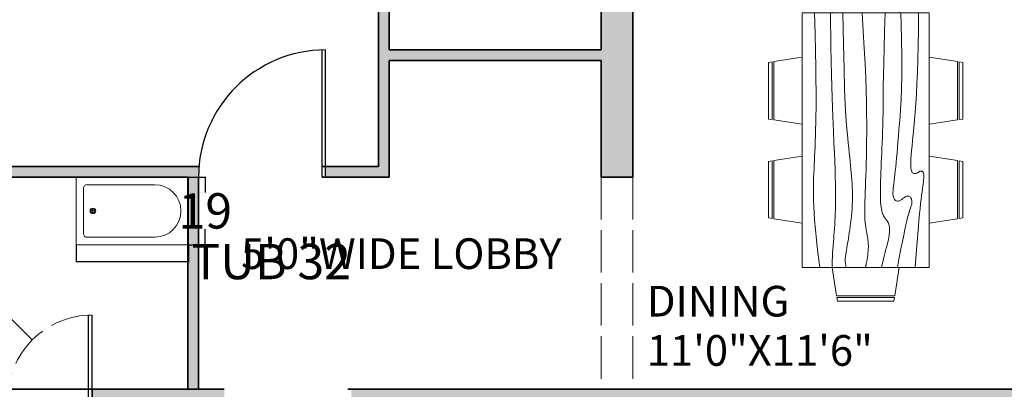
# Model space of a CAD drawing. Units: inches. Extents: x 215 to 969, y -612 to 418.
# Tile 6 of 8: x 405 to 684, y 109 to 214. Entities that reach past the tile are written whole.
import ezdxf

# ---------------------------------------------------------------- set-up
doc = ezdxf.new("R2010")
doc.units = ezdxf.units.IN
doc.header["$MEASUREMENT"] = 0
doc.linetypes.add('ACAD_ISO02W100', pattern=[15, 12, -3])
for name, color, linetype, lineweight in [('A-ANNO-DIMS', 2, 'Continuous', 18), ('A-AREA-IDEN', 7, 'Continuous', 18), ('A-DOOR', 3, 'Continuous', 25), ('A-DOOR-SWNG', 3, 'ACAD_ISO02W100', 13), ('A-FLOR-FIXT', 9, 'Continuous', 18), ('A-FURN', 8, 'Continuous', 18), ('A-WALL', 7, 'Continuous', 35), ('A-WALL-OVHD', 7, 'ACAD_ISO02W100', 18)]:
    doc.layers.add(name, color=color, linetype=linetype, lineweight=lineweight)
doc.layers.add('A-WALL-PATT', color=252, linetype='Continuous', lineweight=13, true_color=0x939598)
doc.styles.get("Standard").update_dxf_attribs({"font": 'arial.ttf'})
doc.dimstyles.get("Standard").update_dxf_attribs({"dimtxt": 10, "dimasz": 0.18, "dimexe": 0.18, "dimexo": 0.0625, "dimgap": 0.09, "dimtad": 0, "dimtih": 1, "dimtoh": 1, "dimdec": 0, "dimzin": 0, "dimdsep": 46, "dimlunit": 3, "dimtxsty": 'Standard', "dimcen": 0.09, "dimadec": 0, "dimazin": 0, "dimtfac": 1, "dimtdec": 0, "dimtofl": 0, "dimtmove": 0, "dimatfit": 3, "dimfxl": 1, "dimtolj": 1, "dimtzin": 0, "dimarcsym": 0})

# ---------------------------------------------------------------- blocks, each defined once
blk = doc.blocks.new('Dining Set - 36 x 72 in.')
for p, q in [((-22.2343, 26.00059), (-23.4847, 17.99762)), ((-22.2304, 26), (-5.7608, 26)), ((-22, 27.5), (-22.1562, 26.50042)), ((-5.8416, 26.5), (-22.1534, 26.5)), ((-22, 27.5), (-6, 27.5)), ((-5.8437, 26.49966), (-6, 27.5)), ((-4.5152, 17.99762), (-5.7655, 25.99926)), ((5.7657, 26.00059), (4.5153, 17.99762)), ((5.7696, 26), (22.2392, 26)), ((6, 27.5), (5.8438, 26.50042)), ((22.1584, 26.5), (5.8466, 26.5)), ((6, 27.5), (22, 27.5)), ((22.1563, 26.49966), (22, 27.5)), ((23.4848, 17.99762), (22.2345, 25.99926)), ((36, 18), (-36, 18)), ((-36, 18), (-36, -18)), ((36, -18), (36, 18)), ((-44.0006, 8.23428), (-35.9976, 9.48474)), ((44.0006, 8.23428), (35.9976, 9.48474)), ((-45.5, 8), (-44.5004, 8.15617)), ((-45.5, 8), (-45.5, -8)), ((-44.5, -8.15843), (-44.5, 8.15338)), ((-44, 8.23041), (-44, -8.23915)), ((44, 8.23041), (44, -8.23915)), ((44.5, -8.15843), (44.5, 8.15338)), ((45.5, 8), (44.5005, 8.15617)), ((45.5, 8), (45.5, -8)), ((-44.4997, -8.15631), (-45.5, -8)), ((-35.9976, -9.48476), (-43.9993, -8.2345)), ((35.9976, -9.48476), (43.9993, -8.2345)), ((44.4997, -8.15631), (45.5, -8)), ((-36, -18), (36, -18)), ((-22.2343, -26.0006), (-23.4847, -17.99762)), ((-4.5152, -17.99762), (-5.7655, -25.99928)), ((5.7657, -26.0006), (4.5153, -17.99762)), ((23.4848, -17.99762), (22.2345, -25.99928)), ((-22.2304, -26), (-5.7608, -26)), ((-22, -27.5), (-22.1562, -26.50044)), ((-5.8416, -26.5), (-22.1534, -26.5)), ((-22, -27.5), (-6, -27.5)), ((-5.8437, -26.49967), (-6, -27.5)), ((5.7696, -26), (22.2392, -26)), ((6, -27.5), (5.8438, -26.50044)), ((22.1584, -26.5), (5.8466, -26.5)), ((6, -27.5), (22, -27.5)), ((22.1563, -26.49967), (22, -27.5))]:
    blk.add_line(p, q)
for points in [[(-36, 15), (-31.1772, 14.97754), (-26.8079, 14.91406), (-22.8538, 14.81543), (-19.276, 14.6875), (-16.0362, 14.53613), (-13.0957, 14.36718), (-10.4159, 14.18652), (-7.9583, 14), (-5.6904, 13.81315), (-3.6035, 13.63021), (-1.6954, 13.45508), (0.0365, 13.29166), (1.5945, 13.14388), (2.9811, 13.01562), (4.1988, 12.9108), (5.25, 12.83333), (6.1393, 12.78613), (6.8802, 12.76823), (7.4883, 12.77767), (7.9792, 12.8125), (8.3685, 12.87077), (8.6719, 12.95052), (8.9049, 13.0498), (9.0833, 13.16666), (9.2205, 13.29899), (9.3216, 13.44401), (9.3895, 13.59879), (9.4271, 13.76041), (9.4373, 13.92594), (9.4232, 14.09245), (9.3875, 14.257), (9.3333, 14.41666), (9.2638, 14.56917), (9.1836, 14.71484), (9.0975, 14.85465), (9.0104, 14.98958), (8.9272, 15.1206), (8.8529, 15.2487), (8.7922, 15.37483), (8.75, 15.5), (8.7305, 15.62467), (8.7344, 15.74739), (8.7617, 15.86621), (8.8125, 15.97916), (8.8867, 16.08431), (8.9844, 16.17968), (9.1055, 16.26334), (9.25, 16.33333), (9.4189, 16.38802), (9.6172, 16.42708), (9.8506, 16.45052), (10.125, 16.45833), (10.4463, 16.45052), (10.8203, 16.42708), (11.2529, 16.38802), (11.75, 16.33333), (12.3184, 16.26318), (12.9694, 16.17838), (13.7151, 16.07991), (14.5677, 15.96875), (15.5395, 15.84586), (16.6426, 15.71224), (17.8893, 15.56884), (19.2917, 15.41666), (20.859, 15.25667), (22.5879, 15.08984), (24.4721, 14.91715), (26.5052, 14.73958), (28.6809, 14.5581), (30.9929, 14.3737), (33.4347, 14.18733), (36, 14)], [(-36, 10), (-28.9766, 10.14274), (-23.1725, 10.20442), (-18.4241, 10.19775), (-14.5677, 10.13541), (-11.4399, 10.03011), (-8.877, 9.89453), (-6.7154, 9.74137), (-4.7917, 9.58333), (-2.9698, 9.43082), (-1.2246, 9.28515), (0.4415, 9.14534), (2.026, 9.01041), (3.5266, 8.87939), (4.9408, 8.7513), (6.266, 8.62516), (7.5, 8.5), (8.6411, 8.37549), (9.6914, 8.2539), (10.6538, 8.13818), (11.5312, 8.03125), (12.3267, 7.93603), (13.043, 7.85547), (13.6831, 7.79248), (14.25, 7.75), (14.7471, 7.7303), (15.1797, 7.73307), (15.5537, 7.75732), (15.875, 7.80208), (16.1494, 7.86637), (16.3828, 7.94922), (16.5811, 8.04964), (16.75, 8.16666), (16.8944, 8.29915), (17.0143, 8.44531), (17.1089, 8.60319), (17.1771, 8.77083), (17.218, 8.94629), (17.2305, 9.1276), (17.2137, 9.31282), (17.1667, 9.5), (17.0895, 9.6875), (16.987, 9.875), (16.8649, 10.0625), (16.7292, 10.25), (16.5856, 10.4375), (16.4401, 10.625), (16.2985, 10.8125), (16.1667, 11), (16.05, 11.18733), (15.9518, 11.3737), (15.8752, 11.5581), (15.8229, 11.73958), (15.798, 11.91715), (15.8034, 12.08984), (15.842, 12.25667), (15.9167, 12.41666), (16.0295, 12.56836), (16.1784, 12.70833), (16.3605, 12.83268), (16.5729, 12.9375), (16.8127, 13.01888), (17.0768, 13.07291), (17.3625, 13.0957), (17.6667, 13.08333), (17.9894, 13.03312), (18.3418, 12.94726), (18.7382, 12.82918), (19.1927, 12.68229), (19.7195, 12.51001), (20.3327, 12.31575), (21.0465, 12.10294), (21.875, 11.875), (22.8357, 11.63354), (23.959, 11.37304), (25.2786, 11.08618), (26.8282, 10.76562), (28.6414, 10.40405), (30.752, 9.99414), (33.1936, 9.52856), (36, 9)], [(-36, 5.5), (-30.7157, 5.3348), (-26.069, 5.20963), (-21.9946, 5.11767), (-18.4271, 5.05208), (-15.3009, 5.00602), (-12.5508, 4.97265), (-10.1112, 4.94515), (-7.9167, 4.91666), (-5.909, 4.88167), (-4.0586, 4.83984), (-2.3429, 4.79215), (-0.7396, 4.73958), (0.7739, 4.6831), (2.22, 4.6237), (3.6213, 4.56233), (5, 4.5), (6.373, 4.43782), (7.7344, 4.3776), (9.0723, 4.32129), (10.375, 4.27083), (11.6309, 4.22819), (12.8281, 4.19531), (13.9551, 4.17415), (15, 4.16666), (15.954, 4.17448), (16.819, 4.19791), (17.6001, 4.23698), (18.3021, 4.29166), (18.9299, 4.36198), (19.4883, 4.44791), (19.9823, 4.54948), (20.4167, 4.66666), (20.7969, 4.79899), (21.1302, 4.94401), (21.4245, 5.09879), (21.6875, 5.26041), (21.9271, 5.42594), (22.1511, 5.59245), (22.3672, 5.757), (22.5834, 5.91666), (22.8065, 6.06868), (23.0404, 6.21093), (23.2879, 6.34147), (23.5521, 6.45833), (23.8358, 6.55957), (24.142, 6.64323), (24.4735, 6.70735), (24.8334, 6.75), (25.2235, 6.76969), (25.642, 6.76692), (26.0858, 6.74267), (26.5521, 6.69791), (27.0379, 6.63362), (27.5404, 6.55078), (28.0565, 6.45036), (28.5834, 6.33333), (29.1242, 6.19987), (29.7071, 6.04687), (30.3661, 5.87044), (31.1354, 5.66666), (32.0493, 5.43164), (33.142, 5.16146), (34.4475, 4.85221), (36, 4.5)], [(-36, -1), (-30.7915, -0.6591), (-26.0195, -0.38216), (-21.6519, -0.16284), (-17.6563, 0.00521), (-14.0005, 0.12833), (-10.6523, 0.21289), (-7.5796, 0.26522), (-4.75, 0.29166), (-2.134, 0.29793), (0.2878, 0.28711), (2.5317, 0.26163), (4.6146, 0.22396), (6.5529, 0.17651), (8.3633, 0.12174), (10.0623, 0.06209), (11.6667, 0), (13.1899, -0.06201), (14.6341, -0.1211), (15.9982, -0.17432), (17.2813, -0.21875), (18.4823, -0.25147), (19.6003, -0.26953), (20.6343, -0.27002), (21.5834, -0.25), (22.4481, -0.20768), (23.2357, -0.14584), (23.9549, -0.06836), (24.6146, 0.02083), (25.2235, 0.11784), (25.7904, 0.21875), (26.3241, 0.31966), (26.8334, 0.41666), (27.3265, 0.50618), (27.8099, 0.58593), (28.2894, 0.65397), (28.7709, 0.70833), (29.2601, 0.74707), (29.763, 0.76823), (30.2855, 0.76985), (30.8334, 0.75), (31.4088, 0.70784), (31.9994, 0.64713), (32.589, 0.57275), (33.1615, 0.48958), (33.7008, 0.4025), (34.1908, 0.3164), (34.6153, 0.23616), (34.9584, 0.16666), (35.2099, 0.11165), (35.3848, 0.07031), (35.504, 0.04069), (35.5886, 0.02083), (35.6594, 0.00879), (35.7377, 0.0026), (35.8442, 0.00032), (36, 0)], [(-36, -6.5), (-27.1843, -6.31267), (-20.084, -6.1263), (-14.469, -5.9419), (-10.1094, -5.76042), (-6.7752, -5.58285), (-4.2363, -5.41016), (-2.2629, -5.24333), (-0.625, -5.08334), (0.8708, -4.93099), (2.2715, -4.78646), (3.5872, -4.64974), (4.8281, -4.52084), (6.0046, -4.39974), (7.127, -4.28646), (8.2053, -4.18099), (9.25, -4.08334), (10.2705, -3.99382), (11.2734, -3.91407), (12.2647, -3.84603), (13.25, -3.79167), (14.2354, -3.75293), (15.2266, -3.73177), (16.2295, -3.73015), (17.25, -3.75), (18.2912, -3.79248), (19.3451, -3.85547), (20.4009, -3.93604), (21.4479, -4.03125), (22.4754, -4.13819), (23.4727, -4.25391), (24.4289, -4.37549), (25.3334, -4.5), (26.1785, -4.62492), (26.9694, -4.74935), (27.7145, -4.87281), (28.4219, -4.99479), (29.1, -5.11483), (29.7572, -5.23242), (30.4016, -5.34709), (31.0417, -5.45834), (31.6837, -5.56437), (32.3262, -5.65821), (32.9658, -5.73153), (33.599, -5.77604), (34.2224, -5.78345), (34.8327, -5.74545), (35.4264, -5.65373), (36, -5.5)], [(-36, -10), (-26.4022, -9.81299), (-18.4675, -9.62891), (-11.9839, -9.45069), (-6.7396, -9.28125), (-2.5226, -9.12354), (0.8789, -8.98047), (3.6769, -8.85498), (6.0833, -8.75), (8.2767, -8.66765), (10.3021, -8.60677), (12.1712, -8.56543), (13.8958, -8.54167), (15.4876, -8.53353), (16.9583, -8.53907), (18.3197, -8.55632), (19.5834, -8.58334), (20.7616, -8.61841), (21.8685, -8.66081), (22.9188, -8.71004), (23.9271, -8.76563), (24.9081, -8.82707), (25.8763, -8.89388), (26.8465, -8.96558), (27.8334, -9.04167), (28.8474, -9.12118), (29.8828, -9.20117), (30.93, -9.27824), (31.9792, -9.34896), (33.0205, -9.40991), (34.0443, -9.45768), (35.0407, -9.48885), (36, -9.5)], [(-36, -14.5), (-30.0881, -14.33513), (-25.0332, -14.21224), (-20.7312, -14.12647), (-17.0781, -14.07292), (-13.97, -14.04671), (-11.3027, -14.04297), (-8.9724, -14.05681), (-6.875, -14.08334), (-4.9224, -14.11833), (-3.0905, -14.16016), (-1.3709, -14.20785), (0.2448, -14.26042), (1.7647, -14.3169), (3.1973, -14.3763), (4.5507, -14.43767), (5.8333, -14.5), (7.0554, -14.5621), (8.235, -14.62175), (9.3922, -14.67652), (10.5469, -14.72396), (11.7192, -14.76164), (12.929, -14.78711), (14.1965, -14.79794), (15.5417, -14.79167), (16.9933, -14.76424), (18.6152, -14.70508), (20.4804, -14.60197), (22.6615, -14.44271), (25.2312, -14.21509), (28.2624, -13.9069), (31.8277, -13.50594), (36, -13)]]:
    blk.add_lwpolyline(points)
blk = doc.blocks.new('Bath Tub - 26 x 60 in.')
for p, q in [((8, -18), (10, -18)), ((9, -17), (9, -19))]:
    blk.add_line(p, q)
blk.add_lwpolyline([(0, -36), (0, 0), (60, 0), (60, -36)], close=True)
for points in [[(6, -4), (42, -4)], [(4, -30), (4, -6)], [(42, -32), (6, -32)]]:
    blk.add_lwpolyline(points)
for radius in [1.5, 1]:
    blk.add_circle((9, -18), radius)
for centre, radius, start, end in [((5.75, -5.75), 1.77, 81.8699, 188.1301), ((42, -18), 14, 270, 90), ((5.75, -30.25), 1.77, 171.8699, 278.1301)]:
    blk.add_arc(centre, radius, start, end)
blk = doc.blocks.new('DOOR-SINGLE-36')
for p, q in [((35, 0), (35, 36)), ((36, 0), (36, 36)), ((35, 0), (36, 0))]:
    blk.add_line(p, q)
blk.add_arc((36, 0), 36, 90, 180)
blk = doc.blocks.new('*D31')
at = {"layer": 'A-ANNO-DIMS', "color": 0, "lineweight": -2, "transparency": 16777216}
for p, q in [((420.68, 150.06), (420.68, 145.17)), ((452.5, 150.06), (452.5, 145.17)), ((420.86, 145.35), (452.32, 145.35)), ((452.5, 145.35), (452.68, 145.35))]:
    blk.add_line(p, q, dxfattribs=at)
at = {"layer": 'A-ANNO-DIMS', "color": 0, "transparency": 16777216}
for points in [[(420.86, 145.38), (420.86, 145.32), (420.68, 145.35)], [(452.32, 145.38), (452.32, 145.32), (452.5, 145.35)]]:
    blk.add_solid(points, dxfattribs=at)
at = {"layer": 'Defpoints', "color": 0, "transparency": 16777216}
for p in [(420.68, 150.12), (452.5, 150.12), (452.5, 145.35)]:
    blk.add_point(p, dxfattribs=at)
at = {"layer": 'A-ANNO-DIMS', "color": 0, "transparency": 16777216, "insert": (475.92, 145.35), "char_height": 10, "attachment_point": 5}
blk.add_mtext('\\A1;TUB 32', dxfattribs=at)
blk = doc.blocks.new('*D32')
at = {"layer": 'A-ANNO-DIMS', "color": 0, "lineweight": -2, "transparency": 16777216}
for p, q in [((452.57, 169.21), (457.46, 169.21)), ((457.28, 169.03), (457.28, 164.86)), ((457.28, 150.3), (457.28, 154.47)), ((452.57, 150.12), (457.46, 150.12))]:
    blk.add_line(p, q, dxfattribs=at)
at = {"layer": 'A-ANNO-DIMS', "color": 0, "transparency": 16777216}
for points in [[(457.25, 169.03), (457.31, 169.03), (457.28, 169.21)], [(457.25, 150.3), (457.31, 150.3), (457.28, 150.12)]]:
    blk.add_solid(points, dxfattribs=at)
at = {"layer": 'Defpoints', "color": 0, "transparency": 16777216}
for p in [(452.5, 169.21), (457.28, 169.21), (452.5, 150.12)]:
    blk.add_point(p, dxfattribs=at)
at = {"layer": 'A-ANNO-DIMS', "color": 0, "transparency": 16777216, "insert": (457.28, 159.67), "char_height": 10, "attachment_point": 5}
blk.add_mtext('\\A1;19', dxfattribs=at)
blk = doc.blocks.new('*D76')
at = {"layer": 'A-ANNO-DIMS', "color": 0, "lineweight": -2, "transparency": 16777216}
for p, q in [((569.29, 365.5), (243.77, 365.5)), ((243.95, 365.32), (243.95, -91.71)), ((243.95, -559.13), (243.95, -102.1)), ((454.66, -559.31), (243.77, -559.31))]:
    blk.add_line(p, q, dxfattribs=at)
at = {"layer": 'A-ANNO-DIMS', "color": 0, "transparency": 16777216}
for points in [[(243.92, 365.32), (243.98, 365.32), (243.95, 365.5)], [(243.92, -559.13), (243.98, -559.13), (243.95, -559.31)]]:
    blk.add_solid(points, dxfattribs=at)
at = {"layer": 'Defpoints', "color": 0, "transparency": 16777216}
for p in [(569.35, 365.5), (243.95, -559.31), (454.72, -559.31)]:
    blk.add_point(p, dxfattribs=at)
at = {"layer": 'A-ANNO-DIMS', "color": 0, "transparency": 16777216, "insert": (243.95, -96.91), "char_height": 10, "attachment_point": 5}
blk.add_mtext('\\A1;924.8', dxfattribs=at)
blk = doc.blocks.new('*D85')
at = {"layer": 'A-ANNO-DIMS', "color": 0, "lineweight": -2, "transparency": 16777216}
for p, q in [((397.96, 133.26), (398.14, 133.26)), ((398.14, 133.26), (408.16, 123.3)), ((425.11, 106.37), (425.29, 106.37)), ((425.2, 106.28), (425.2, 106.46))]:
    blk.add_line(p, q, dxfattribs=at)
at = {"layer": 'A-ANNO-DIMS', "color": 0, "transparency": 16777216}
blk.add_solid([(408.18, 123.32), (408.14, 123.28), (408.29, 123.18)], dxfattribs=at)
at = {"layer": 'Defpoints', "color": 0, "transparency": 16777216}
for p in [(408.29, 123.18), (425.2, 106.37)]:
    blk.add_point(p, dxfattribs=at)
at = {"layer": 'A-ANNO-DIMS', "color": 0, "transparency": 16777216, "insert": (372.32, 133.26), "char_height": 10, "attachment_point": 5}
blk.add_mtext('\\A1;R23.847', dxfattribs=at)

msp = doc.modelspace()

# ---------------------------------------------------------------- hatches: boundary and pattern name
at = {"layer": 'A-WALL-PATT'}
h = msp.add_hatch(color=256, dxfattribs=at)
h.dxf.hatch_style = 1
h.paths.add_polyline_path([(764.0736, 322.2135), (569.3535, 322.2135), (565.0643, 322.2135), (565.0643, 313.2135), (569.3535, 313.2135), (569.3535, 205.2135), (509.3535, 205.2135), (509.3535, 247.2592), (506.3535, 247.2592), (506.3535, 172.2135), (491.3535, 172.2135), (491.3535, 169.2135), (509.3535, 169.2135), (509.3535, 202.2135), (569.3535, 202.2135), (569.3535, 169.2135), (578.3535, 169.2135), (578.3535, 205.2135), (578.3535, 237.2135), (615.7789, 237.2135), (615.7789, 246.2135), (578.3535, 246.2135), (578.3535, 313.2135), (710.3535, 313.2135), (710.3535, 246.2135), (710.3535, 211.3874), (719.3535, 211.3874), (719.3535, 295.2135), (719.3535, 313.2135), (764.0736, 313.2135)])
h.paths.add_polyline_path([(879.3535, 322.2135), (811.6486, 322.2135), (811.6486, 313.2135), (870.3535, 313.2135), (870.3535, 215.3905, -0.06325422), (879.3535, 216.5337), (879.3535, 313.2135)])
h.paths.add_polyline_path([(879.3535, 157.2135), (879.3535, 180.5337), (870.3535, 180.5337), (870.3535, 157.2135), (719.3535, 157.2135), (710.3535, 157.2135), (710.3535, 148.2135), (719.3535, 148.2135), (870.3535, 148.2135), (870.3535, 16.2135), (838.4933, 16.2135), (838.4933, 13.2135), (870.3535, 13.2135), (870.3535, -37.7865), (844.0345, -37.7865), (844.0345, -46.7865), (870.3535, -46.7865), (879.3535, -46.7865), (879.3535, -37.7865), (879.3535, 137.613)])
h.paths.add_polyline_path([(710.3535, 246.2135), (663.4146, 246.2135), (663.4146, 237.2135), (710.3535, 237.2135)], flags=17)
h.paths.add_polyline_path([(541.2942, 322.2135), (509.3535, 322.2135), (468.3222, 322.2135), (468.3222, 313.2135), (500.3535, 313.2135), (509.3535, 313.2135), (541.2942, 313.2135)])
h.paths.add_polyline_path([(509.3535, 313.2135), (503.3535, 313.2135), (503.3535, 277.5241, -0.04952579), (509.3535, 277.4203)], flags=17)
h.paths.add_polyline_path([(420.2828, 322.2135), (335.3535, 322.2135), (335.3535, 235.2487), (344.3535, 235.2487), (344.3535, 284.1885), (344.3535, 313.2135), (420.2828, 313.2135)])
h.paths.add_polyline_path([(335.3535, 181.2135), (290.3535, 181.2135), (290.3535, 103.2135), (335.3535, 103.2135), (335.3535, 112.2135), (299.3535, 112.2135), (299.3535, 129.1615), (299.3535, 172.2135), (335.3535, 172.2135)])
h.paths.add_polyline_path([(344.3535, 199.3097), (335.3535, 199.3097), (335.3535, 172.2135), (335.3535, 157.3369), (344.3535, 157.3369), (344.3535, 169.2135), (452.3535, 169.2135), (452.5037, 169.2135), (452.5037, 150.1199), (452.3535, 109.2135), (455.3535, 109.2135), (455.3535, 169.2135, -0.02086055), (455.4787, 172.2135), (344.3535, 172.2135)])
h.paths.add_polyline_path([(344.3535, 133.3441), (335.3535, 133.3441), (335.3535, 77.89), (344.3535, 77.89), (344.3535, 103.2135), (401.3556, 103.2135), (401.3556, 109.2135), (344.3535, 109.2135)])
h.paths.add_polyline_path([(462.6362, 109.2135), (443.0437, 109.2135), (425.2018, 109.2135), (425.2018, 106.2135), (452.3535, 106.2135), (462.7615, 106.2135, -0.02086055)])
h.paths.add_polyline_path([(540.3535, 106.2135), (684.3535, 106.2135), (684.3535, 35.7135), (687.3535, 35.7135), (687.3535, 56.1856), (693.3535, 56.1856), (693.3535, 109.2135), (540.3535, 109.2135), (531.3535, 109.2135), (498.6362, 109.2135), (498.6362, 106.2135), (531.3535, 106.2135), (531.3535, -37.7865), (507.9524, -37.7865), (507.9524, -46.7865), (610.6038, -46.7865), (610.6038, -37.7865), (540.3535, -37.7865)])
h.paths.add_polyline_path([(578.3535, 358.6622), (555.879, 358.6622), (555.879, 349.6622), (569.3535, 349.6622), (569.3535, 322.2135), (578.3535, 322.2135)])
h.paths.add_polyline_path([(525.962, 358.6622), (503.3535, 358.6622), (503.3535, 322.2135), (509.3535, 322.2135), (509.3535, 349.6622), (525.962, 349.6622)])
h.paths.add_polyline_path([(344.3535, 30.022), (335.3535, 30.022), (335.3535, -37.7865), (335.3535, -46.7865), (484.3302, -46.7865), (484.3302, -37.7865), (344.3535, -37.7865)])
h.paths.add_polyline_path([(719.1188, -37.7865), (698.4193, -37.7865), (693.3535, -37.7865), (693.3535, 7.424, -0.07717369), (684.3535, 6.0404), (684.3535, -37.7865), (658.8269, -37.7865), (658.8269, -46.7865), (684.3535, -46.7865), (684.3535, -82.7865), (693.3535, -82.7865), (704.1236, -82.7865), (704.1236, -78.0462), (693.3535, -78.0462), (693.3535, -46.7865), (719.1188, -46.7865)])
h.paths.add_polyline_path([(684.3535, -14.2202), (669.6716, -14.2202), (669.6716, -16.6044, -0.23606798), (667.6716, -17.6044), (667.6716, -18.6044, -0.11764706), (650.6716, -18.6044), (650.6716, -17.6044, -0.23606798), (648.6716, -16.6044), (648.6716, -14.2202), (603.0565, -14.2202), (603.0565, -37.7865), (684.3535, -37.7865)], flags=17)
h.paths.add_polyline_path([(665.6716, -14.2202), (652.6716, -14.2202), (652.6716, -16.6044, -0.23606798), (650.6716, -17.6044), (650.6716, -18.6044, 0.11764706), (667.6716, -18.6044), (667.6716, -17.6044, -0.23606798), (665.6716, -16.6044)], flags=16)
h.paths.add_polyline_path([(786.7385, -37.7865), (755.3535, -37.7865), (755.3535, 13.2135), (769.0808, 13.2135), (769.0808, 16.2135), (755.3535, 16.2135), (755.3535, 73.2135), (753.3535, 73.2135), (693.3535, 73.2135), (693.3535, 70.2135), (753.3535, 70.2135), (753.3535, -37.7865), (743.3062, -37.7865), (743.3062, -46.7865), (781.7385, -46.7865), (781.7385, -82.7865), (786.7385, -82.7865), (786.7385, -82.3744), (786.7385, -46.7865)])
h.paths.add_polyline_path([(844.0345, -37.7865), (786.7385, -37.7865), (786.7385, -46.7865), (844.0345, -46.7865)], flags=17)
h.paths.add_polyline_path([(781.7385, -78.0462), (704.1236, -78.0462), (704.1236, -82.7865), (781.7385, -82.7865)], flags=17)
h.paths.add_polyline_path([(344.3535, -46.7865), (335.3535, -46.7865), (335.3535, -166.4525), (344.3535, -166.4525)])
h.paths.add_polyline_path([(382.6632, 103.2135), (344.3535, 103.2135), (344.3535, 77.89), (344.3535, 32.7135), (363.5083, 32.7135), (382.6632, 32.7135)])
h.paths.add_polyline_path([(879.3535, -46.7865), (870.3535, -46.7865), (870.3535, -166.4525), (879.3535, -166.4525)])
h.paths.add_polyline_path([(879.3535, -166.4525), (799.4745, -166.4525), (799.4745, -175.4525), (855.3535, -175.4525), (870.3535, -175.4525), (870.3535, -192.5449), (879.3535, -192.5449), (879.3535, -175.4525)])
h.paths.add_polyline_path([(763.1775, -166.4525), (655.7214, -166.4525), (655.7214, -175.4525), (763.1775, -175.4525)])
h.paths.add_polyline_path([(619.8538, -166.4525), (550.8369, -166.4525), (550.8369, -175.4525), (619.8538, -175.4525)])
h.paths.add_polyline_path([(527.1282, -166.4525), (427.0819, -166.4525), (427.0819, -175.4525), (527.1282, -175.4525)])
h.paths.add_polyline_path([(391.4021, -166.4525), (335.3535, -166.4525), (335.3535, -175.4525), (335.3535, -236.0109), (344.3535, -236.0109), (344.3535, -187.5037), (344.3535, -175.4525), (391.4021, -175.4525)])
h.paths.add_polyline_path([(344.3535, -271.9249), (335.3535, -271.9249), (335.3535, -331.0209), (344.3535, -331.0209), (344.3535, -314.4525), (412.4218, -314.4525, -0.02503209), (412.3073, -311.4525), (344.3535, -311.4525)])
h.paths.add_polyline_path([(470.1954, -311.4525), (442.3073, -311.4525), (442.3073, -314.4525), (470.0702, -314.4525, -0.02086055)])
h.paths.add_polyline_path([(455.3535, -314.4525), (452.3535, -314.4525), (452.3535, -374.4525), (455.3535, -374.4525)])
h.paths.add_polyline_path([(579.3535, -241.4072), (519.3535, -241.4072), (519.3535, -283.4525), (579.3535, -283.4525)])
h.paths.add_polyline_path([(516.5043, -281.1089), (584.3098, -281.1089), (584.3098, -264.0138), (516.5043, -264.0138)], flags=9)
h.paths.add_polyline_path([(516.4662, -263.2183), (581.1504, -263.2183), (581.1504, -245.8948), (516.4662, -245.8948)], flags=9)

# ---------------------------------------------------------------- linework, layer by layer
at = {"layer": 'A-DOOR'}
for p, q in [((424.2018, 106.2135), (424.2018, 130.2135)), ((425.2018, 106.2135), (425.2018, 130.2135)), ((425.2018, 109.2135), (425.2018, 106.2135))]:
    msp.add_line(p, q, dxfattribs=at)
at = {"layer": 'A-DOOR-SWNG'}
msp.add_arc((425.2018, 106.3669), 23.8466, 90, 180.368506, dxfattribs=at)
at = {"layer": 'A-WALL'}
for p, q in [((509.3535, 205.2135), (509.3535, 313.2135)), ((569.3535, 313.2135), (569.3535, 205.2135)), ((506.3535, 172.2135), (506.3535, 248.2592)), ((578.3535, 237.2135), (578.3535, 205.2135)), ((569.3535, 205.2135), (509.3535, 205.2135)), ((578.3535, 169.2135), (578.3535, 205.2135)), ((509.3535, 169.2135), (509.3535, 202.2135)), ((569.3535, 202.2135), (509.3535, 202.2135)), ((569.3535, 202.2135), (569.3535, 169.2135)), ((344.3535, 172.2135), (455.4787, 172.2135)), ((490.3535, 172.2135), (506.3535, 172.2135)), ((344.3535, 169.2135), (452.3535, 169.2135)), ((452.3535, 109.2135), (452.3535, 169.2135)), ((455.3535, 109.2135), (455.3535, 169.2135)), ((490.3535, 169.2135), (509.3535, 169.2135)), ((569.3535, 169.2135), (578.3535, 169.2135)), ((344.3535, 109.2135), (452.3535, 109.2135)), ((462.6362, 109.2135), (443.0437, 109.2135)), ((531.3535, 109.2135), (497.6362, 109.2135)), ((531.3535, 109.2135), (543.2726, 109.2135)), ((540.3535, 109.2135), (693.3535, 109.2135))]:
    msp.add_line(p, q, dxfattribs=at)
at = {"layer": 'A-WALL-OVHD'}
for p, q in [((569.3535, 169.2135), (569.3535, 109.2135)), ((578.3535, 169.2135), (578.3535, 109.2135))]:
    msp.add_line(p, q, dxfattribs=at)

# ---------------------------------------------------------------- block references
at = {"layer": 'A-DOOR'}
msp.add_blockref('DOOR-SINGLE-36', (455.353, 169.214), dxfattribs=at)
at = {"layer": 'A-FLOR-FIXT', "xscale": 0.5303784961530699, "yscale": 0.5303784961530699, "zscale": 0.5303784961530699}
msp.add_blockref('Bath Tub - 26 x 60 in.', (420.681, 169.2135), dxfattribs=at)
at = {"layer": 'A-FURN', "rotation": 270}
msp.add_blockref('Dining Set - 36 x 72 in.', (644.2464, 179.6732), dxfattribs=at)

# ---------------------------------------------------------------- texts
at = {"layer": 'A-AREA-IDEN'}
for s, height, p in [('5\'0"WIDE LOBBY', 8.677368, (467.415, 143.2419)), ('DINING', 8.67737, (582.2823, 129.8006)), ('11\'0"X11\'6"', 8.677368, (582.2823, 115.8611))]:
    msp.add_text(s, height=height, dxfattribs=at).set_placement(p)

# ---------------------------------------------------------------- dimensions: what is measured, and where the dimension line sits
at = {"layer": 'A-ANNO-DIMS'}
for base, p1, p2, override, picture, middle in [((243.9535, -559.3132), (569.3535, 365.5008), (454.7218, -559.3132), {"dimdec": 1, "dimlfac": 1, "dimrnd": 0, "dimzin": 0, "dimdsep": 46, "dimlunit": 2}, '*D76', (243.9535, -96.9062)), ((457.2772, 169.2135), (452.5037, 150.1199), (452.5037, 169.2135), {"dimdec": 0, "dimlfac": 1, "dimrnd": 0, "dimzin": 0, "dimdsep": 46, "dimlunit": 2}, '*D32', (457.2772, 159.6667))]:
    dim = msp.add_linear_dim(base=base, p1=p1, p2=p2, angle=90, dimstyle='Standard', override=override, dxfattribs=at)
    dim.commit()
    dim.dimension.update_dxf_attribs({"geometry": picture, "text_midpoint": middle})
dim = msp.add_linear_dim(base=(452.5037, 145.3465), p1=(420.681, 150.1199), p2=(452.5037, 150.1199), text='TUB <>', dimstyle='Standard', override={"dimdec": 0, "dimlfac": 1, "dimrnd": 0, "dimzin": 0, "dimdsep": 46, "dimlunit": 2}, dxfattribs=at)
dim.commit()
dim.dimension.update_dxf_attribs({"geometry": '*D31', "text_midpoint": (475.9218, 145.3465)})
dim = msp.add_radius_dim(center=(425.2018, 106.3669), mpoint=(408.2859, 123.1751), dimstyle='Standard', override={"dimdec": 3, "dimlfac": 1, "dimrnd": 0, "dimzin": 0, "dimdsep": 46, "dimlunit": 2}, dxfattribs=at)
dim.commit()
dim.dimension.update_dxf_attribs({"geometry": '*D85', "text_midpoint": (372.3241, 133.26), "dimtype": 164})

doc.saveas('drawing.dxf')
